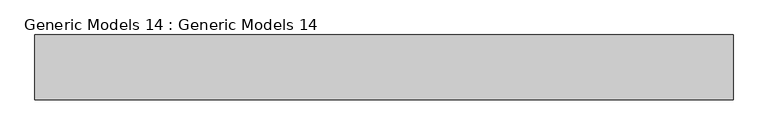
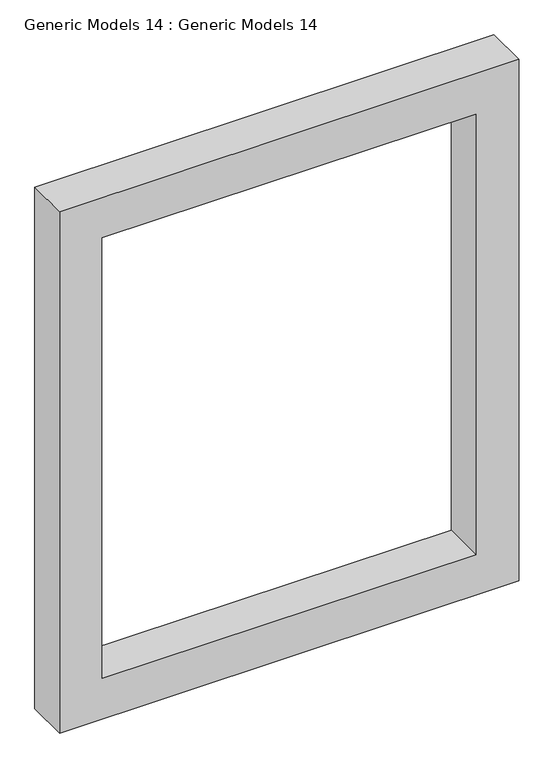
"""IFC4 building model written with IfcOpenShell, lengths in millimetres: proxy geometry, Generic Models 14 : Generic Models 14."""

from ifc_helpers import new_model, si_unit, frame, origin, place, context, project, spatial, polyline, outline, extrude, source, transform, mapped, element, save


def generic_models_14_generic_models_14_14abf339(model_context):
    return source(origin(), model_context, "Body", "SweptSolid", [
        extrude(outline(polyline([(6000.75, -3553.3586008), (4035.4676291, -3553.3586008), (4035.4676291, -1915.0586008), (6000.75, -1915.0586008), (6000.75, -3553.3586008)]), holes=[polyline([(5848.35, -3400.9586008), (5848.35, -2067.4586008), (4187.8676291, -2067.4586008), (4187.8676291, -3400.9586008), (5848.35, -3400.9586008)])]), frame((0.0, 4970.6155883, 0.0), z_axis=(0.0, 1.0, 0.0), x_axis=(0.0, 0.0, 1.0)), (0.0, 0.0, 1.0), 152.4),
    ])


if __name__ == "__main__":
    model = new_model("IFC4")
    model_context = context("Model", 3, world=origin())
    ifc_project = project(units=[si_unit("LENGTHUNIT", "METRE", prefix="MILLI")], contexts=[model_context])
    site = spatial("IfcSite", under=ifc_project)
    building = spatial("IfcBuilding", under=site)
    placement = place(None, origin())
    generic_models_14_generic_models_14_shape = generic_models_14_generic_models_14_14abf339(model_context)
    element("IfcBuildingElementProxy", 1, Name="Generic Models 14 : Generic Models 14", ObjectType="Generic Models 14 : Generic Models 14", at=placement, inside=building, context=model_context, shape_type="MappedRepresentation", body=[
        mapped(generic_models_14_generic_models_14_shape, transform((0.0, 0.0, 0.0), x_axis=(1.0, 0.0, 0.0), y_axis=(0.0, 1.0, 0.0), z_axis=(0.0, 0.0, 1.0))),
    ])
    save(model, "model.ifc")

# Revit data of these elements
# Element 1 (IfcBuildingElementProxy, "Generic Models 14 : Generic Models 14")
#   Materials on its faces: "feature frame"
# Materials
#   "feature frame": class "Generic", colour RGB 120 120 120, transparency 0, Cost = 0
